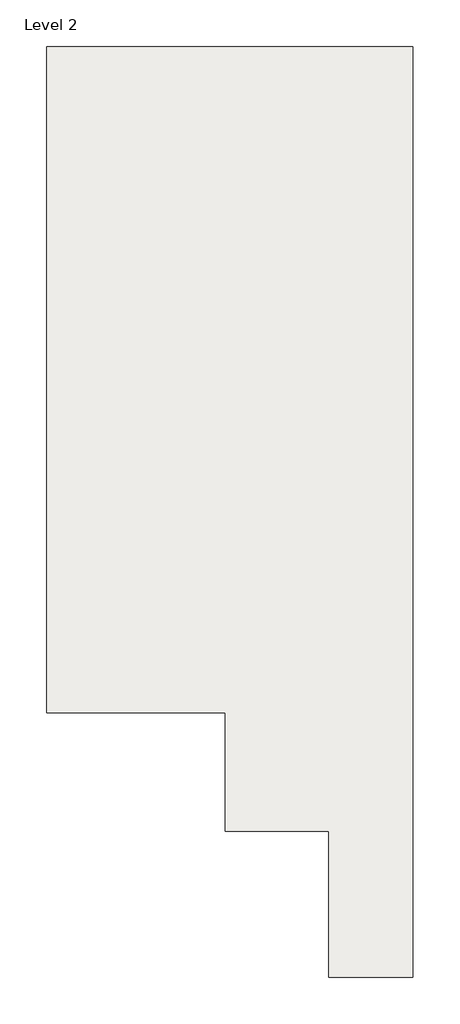
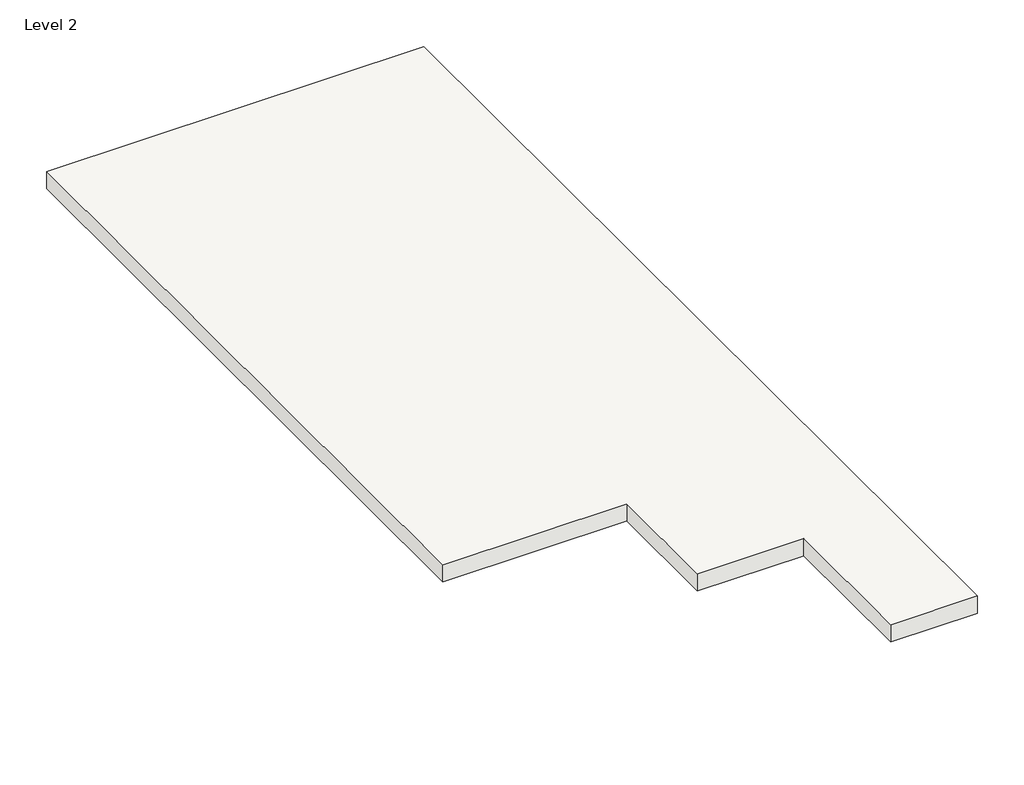
# One storey: 1 roof.
"""IFC4 building model written with IfcOpenShell, lengths in millimetres."""

from ifc_helpers import new_model, si_unit, frame, origin, place, context, project, spatial, polyline, outline, extrude, element, save

model = new_model("IFC4")

# Units and contexts
model_context = context("Model", 3, world=origin())
ifc_project = project(units=[si_unit("LENGTHUNIT", "METRE", prefix="MILLI")], contexts=[model_context])

# Site, building, storey
site = spatial("IfcSite", under=ifc_project)
building = spatial("IfcBuilding", under=site)
storey = spatial("IfcBuildingStorey", under=building, Name="Level 2", Elevation=3048.0)

# Roof
placement = place(None, origin())
element("IfcRoof", 1, ObjectType="Generic - 12\"", at=placement, inside=storey, context=model_context, shape_type="SweptSolid", body=[
    extrude(outline(polyline([(-14717.9112155, 12967.4104001), (-8418.7112155, 12967.4104001), (-8418.7112155, -3034.5895999), (-9866.5112155, -3034.5895999), (-9866.5112155, -519.9895999), (-11644.5112155, -519.9895999), (-11644.5112155, 1512.0104001), (-14717.9112155, 1512.0104001), (-14717.9112155, 12967.4104001)])), frame((0.0, 0.0, 3048.0), z_axis=(0.0, 0.0, 1.0), x_axis=(1.0, 0.0, 0.0)), (0.0, 0.0, 1.0), 304.8),
])

save(model, "model.ifc")

# Revit data of these elements
# Type "Generic - 12\""
#   Assembly Code = "B1020"
#   Layers, outside or top first: 1' - 0" "Brick, Soldier Course" (function 1)
# Element 1 (IfcRoof, "Generic - 12\"")
#   built-in parameter 1001705 = 11 (stored number, unit not read)
#   built-in parameter 1001710 = 33615
#   Phase Created = New Construction
#   Materials on its faces: "Brick, Soldier Course"
# Materials
#   "Brick, Soldier Course": class "Masonry", colour RGB 170 98 104, transparency 0, Description = "Common brick soldier coursed", Cost = 0
